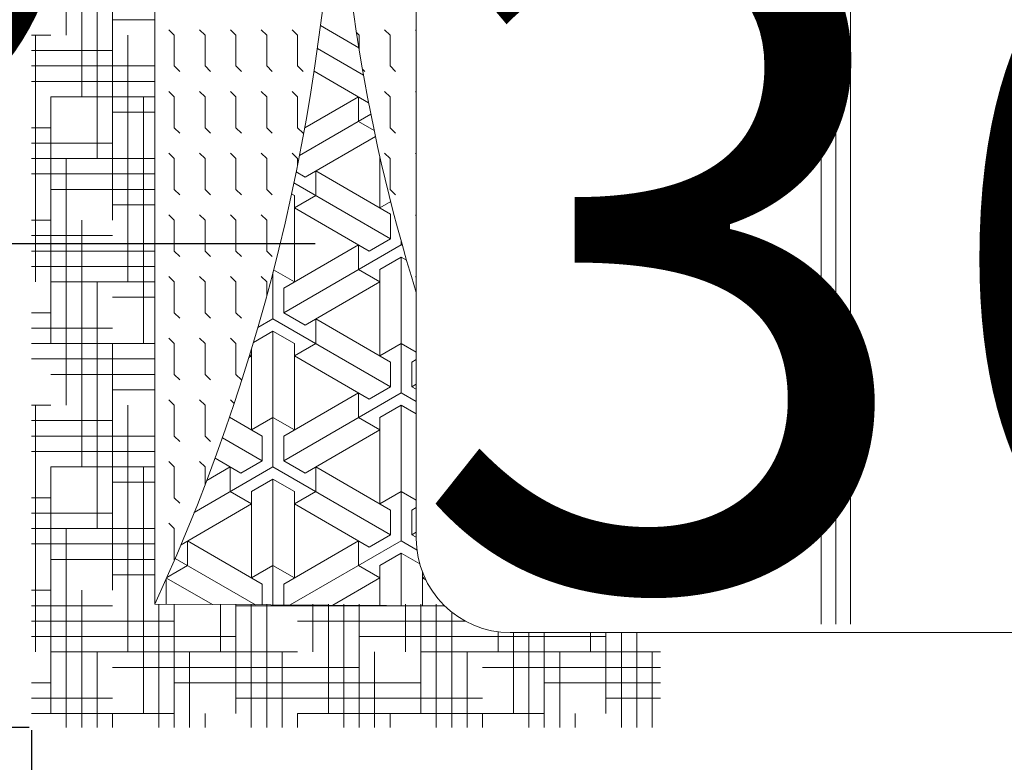
# Model space of a CAD drawing. Units: inches. Extents: x -90 to 536, y -553 to 299.
# Tile 5 of 27: x 96 to 122, y -394 to -375. Entities that reach past the tile are written whole.
import ezdxf

# ---------------------------------------------------------------- set-up
doc = ezdxf.new("R2010")
doc.units = ezdxf.units.IN
doc.layers.add('A-ANNO-DIMS', color=2, linetype='Continuous', lineweight=18)
doc.layers.add('Furniture', color=2, linetype='Continuous', lineweight=18)
doc.styles.get("Standard").update_dxf_attribs({"font": 'arial.ttf'})
doc.dimstyles.get("Standard").update_dxf_attribs({"dimtxt": 18, "dimasz": 12, "dimexe": 0.18, "dimexo": 0.0625, "dimgap": 0.09, "dimtad": 0, "dimtih": 1, "dimtoh": 1, "dimdec": 0, "dimzin": 0, "dimdsep": 46, "dimlunit": 3, "dimtxsty": 'Standard', "dimcen": 0.09, "dimadec": 0, "dimazin": 0, "dimtfac": 1, "dimtdec": 0, "dimtofl": 0, "dimtmove": 0, "dimatfit": 3, "dimfxl": 1, "dimtolj": 1, "dimtzin": 0, "dimarcsym": 0})

# ---------------------------------------------------------------- blocks, each defined once
blk = doc.blocks.new('A$C62731D1C')
for p, q in [((1.46787, 2.14084, 0.68571), (1.46787, 0.38824, 0.68571)), ((0.10613, 0.66415, 0.68571), (1.46095, 0.66415, 0.68571)), ((0.10613, 0.65215, 0.68571), (1.46095, 0.65215, 0.68571)), ((0.10613, 0.64015, 0.68571), (1.46095, 0.64015, 0.68571)), ((1.4835, 0.31577, 0.68571), (1.4835, 0.50998, 0.68571)), ((1.4835, 0.50327, 0.68571), (1.54488, 0.50327, 0.68571)), ((1.496, 0.36577, 0.68571), (1.496, 0.50998, 0.68571)), ((1.5085, 0.41577, 0.68571), (1.5085, 0.50998, 0.68571)), ((1.521, 0.46577, 0.68571), (1.521, 0.50998, 0.68571)), ((1.46787, 0.49077, 0.68571), (1.54488, 0.49077, 0.68571)), ((1.46787, 0.47827, 0.68571), (1.54488, 0.47827, 0.68571)), ((1.46787, 0.46577, 0.68571), (1.5335, 0.46577, 0.68571)), ((1.471, 0.26577, 0.68571), (1.471, 0.46577, 0.68571)), ((1.46787, 0.45327, 0.68571), (1.4835, 0.45327, 0.68571)), ((1.5335, 0.44077, 0.68571), (1.54488, 0.44077, 0.68571)), ((1.4835, 0.42827, 0.68571), (1.54488, 0.42827, 0.68571)), ((1.46787, 0.41577, 0.68571), (1.54488, 0.41577, 0.68571)), ((1.5335, 0.21577, 0.68571), (1.5335, 0.41577, 0.68571)), ((1.46787, 0.40327, 0.68571), (1.54488, 0.40327, 0.68571)), ((1.46787, 0.39077, 0.68571), (1.5335, 0.39077, 0.68571)), ((1.46722, 0.37827, 0.68571), (1.4835, 0.37827, 0.68571)), ((1.521, 0.16577, 0.68571), (1.521, 0.36577, 0.68571)), ((1.5335, 0.36577, 0.68571), (1.54488, 0.36577, 0.68571)), ((1.4585, 0.21577, 0.68571), (1.4585, 0.35163, 0.68571)), ((1.4835, 0.35327, 0.68571), (1.54488, 0.35327, 0.68571)), ((1.45128, 0.34077, 0.68571), (1.54488, 0.34077, 0.68571)), ((1.446, 0.33481, 0.68571), (1.44488, 0.1, 0.68571)), ((1.44488, 0.32827, 0.68571), (1.54488, 0.32827, 0.68571)), ((1.446, 0.16577, 0.68571), (1.446, 0.33481, 0.68571)), ((1.42502, 0.31973, 0.68571), (1.4235, 0.31709, 0.68571)), ((1.39167, 0.31204, 0.68571), (0.17247, 0.31204, 0.68571)), ((0.97908, 0.31135, 0.68571), (0.97977, 0.31204, 0.68571)), ((1.02908, 0.31135, 0.68571), (1.02977, 0.31204, 0.68571)), ((1.07908, 0.31135, 0.68571), (1.07977, 0.31204, 0.68571)), ((1.12908, 0.31135, 0.68571), (1.12977, 0.31204, 0.68571)), ((1.17908, 0.31135, 0.68571), (1.17977, 0.31204, 0.68571)), ((1.2335, 0.29977, 0.68571), (1.24058, 0.31204, 0.68571)), ((1.2485, 0.30843, 0.68571), (1.24642, 0.31204, 0.68571)), ((1.26642, 0.31204, 0.68571), (1.2685, 0.30843, 0.68571)), ((1.2685, 0.30843, 0.68571), (1.27058, 0.31204, 0.68571)), ((1.2735, 0.29977, 0.68571), (1.28058, 0.31204, 0.68571)), ((1.2835, 0.29977, 0.68571), (1.29058, 0.31204, 0.68571)), ((1.3535, 0.29977, 0.68571), (1.36058, 0.31204, 0.68571)), ((1.3685, 0.30843, 0.68571), (1.36642, 0.31204, 0.68571)), ((1.38642, 0.31204, 0.68571), (1.3885, 0.30843, 0.68571)), ((1.3885, 0.30843, 0.68571), (1.39058, 0.31204, 0.68571)), ((1.3935, 0.29977, 0.68571), (1.40091, 0.3126, 0.68571)), ((1.4035, 0.29977, 0.68571), (1.41221, 0.31486, 0.68571)), ((1.41896, 0.31709, 0.68571), (1.44592, 0.31709, 0.68571)), ((1.42263, 0.31861, 0.68571), (1.4235, 0.31709, 0.68571)), ((1.44488, 0.31577, 0.68571), (1.5335, 0.31577, 0.68571)), ((1.5085, 0.11577, 0.68571), (1.5085, 0.31577, 0.68571)), ((1.1635, 0.29977, 0.68571), (1.16604, 0.30418, 0.68571)), ((1.2685, 0.30843, 0.68571), (1.2485, 0.30843, 0.68571)), ((1.3885, 0.30843, 0.68571), (1.3685, 0.30843, 0.68571)), ((1.1535, 0.29977, 0.68571), (1.15051, 0.29977, 0.68571)), ((1.1535, 0.29977, 0.68571), (1.15408, 0.30077, 0.68571)), ((1.1535, 0.29977, 0.68571), (1.2085, 0.20451, 0.68571)), ((1.2735, 0.29977, 0.68571), (1.1635, 0.29977, 0.68571)), ((1.1635, 0.29977, 0.68571), (1.1735, 0.28245, 0.68571)), ((1.2335, 0.29977, 0.68571), (1.2435, 0.28245, 0.68571)), ((1.2735, 0.29977, 0.68571), (1.3285, 0.20451, 0.68571)), ((1.3935, 0.29977, 0.68571), (1.2835, 0.29977, 0.68571)), ((1.2835, 0.29977, 0.68571), (1.2935, 0.28245, 0.68571)), ((1.3535, 0.29977, 0.68571), (1.3635, 0.28245, 0.68571)), ((1.3935, 0.29977, 0.68571), (1.44541, 0.20987, 0.68571)), ((1.44583, 0.29977, 0.68571), (1.4035, 0.29977, 0.68571)), ((1.4035, 0.29977, 0.68571), (1.4135, 0.28245, 0.68571)), ((1.44488, 0.30327, 0.68571), (1.4835, 0.30327, 0.68571)), ((0.97908, 0.28635, 0.68571), (0.9835, 0.29077, 0.68571)), ((0.9835, 0.29077, 0.68571), (1.0085, 0.29077, 0.68571)), ((1.0085, 0.29077, 0.68571), (1.01292, 0.29519, 0.68571)), ((1.02908, 0.28635, 0.68571), (1.0335, 0.29077, 0.68571)), ((1.0335, 0.29077, 0.68571), (1.0585, 0.29077, 0.68571)), ((1.0585, 0.29077, 0.68571), (1.06292, 0.29519, 0.68571)), ((1.07908, 0.28635, 0.68571), (1.0835, 0.29077, 0.68571)), ((1.0835, 0.29077, 0.68571), (1.1085, 0.29077, 0.68571)), ((1.1285, 0.29111, 0.68571), (1.0935, 0.23049, 0.68571)), ((1.10332, 0.21286, 0.68571), (1.1485, 0.29111, 0.68571)), ((1.1085, 0.29077, 0.68571), (1.11292, 0.29519, 0.68571)), ((1.11842, 0.29126, 0.68571), (1.1235, 0.28245, 0.68571)), ((1.1485, 0.29111, 0.68571), (1.1285, 0.29111, 0.68571)), ((1.1485, 0.29111, 0.68571), (1.1585, 0.27379, 0.68571)), ((1.2135, 0.19585, 0.68571), (1.2685, 0.29111, 0.68571)), ((1.2485, 0.29111, 0.68571), (1.2135, 0.23049, 0.68571)), ((1.2685, 0.29111, 0.68571), (1.2485, 0.29111, 0.68571)), ((1.2685, 0.29111, 0.68571), (1.2785, 0.27379, 0.68571)), ((1.3335, 0.19585, 0.68571), (1.3885, 0.29111, 0.68571)), ((1.3685, 0.29111, 0.68571), (1.3335, 0.23049, 0.68571)), ((1.3885, 0.29111, 0.68571), (1.3685, 0.29111, 0.68571)), ((1.3885, 0.29111, 0.68571), (1.3985, 0.27379, 0.68571)), ((1.5335, 0.29077, 0.68571), (1.54488, 0.29077, 0.68571)), ((1.08156, 0.28245, 0.68571), (1.1235, 0.28245, 0.68571)), ((1.1735, 0.26513, 0.68571), (1.1835, 0.28245, 0.68571)), ((1.1735, 0.28245, 0.68571), (1.2435, 0.28245, 0.68571)), ((1.2185, 0.22183, 0.68571), (1.1835, 0.28245, 0.68571)), ((1.2935, 0.26513, 0.68571), (1.3035, 0.28245, 0.68571)), ((1.2935, 0.28245, 0.68571), (1.3635, 0.28245, 0.68571)), ((1.3385, 0.22183, 0.68571), (1.3035, 0.28245, 0.68571)), ((1.4135, 0.26513, 0.68571), (1.4235, 0.28245, 0.68571)), ((1.4135, 0.28245, 0.68571), (1.44575, 0.28245, 0.68571)), ((1.44557, 0.24423, 0.68571), (1.4235, 0.28245, 0.68571)), ((1.03828, 0.2734, 0.68571), (1.01275, 0.2292, 0.68571)), ((1.04766, 0.27525, 0.68571), (1.08108, 0.21737, 0.68571)), ((1.0535, 0.26513, 0.68571), (1.06091, 0.27796, 0.68571)), ((1.0985, 0.22183, 0.68571), (1.06553, 0.27894, 0.68571)), ((1.1585, 0.27379, 0.68571), (1.1235, 0.21317, 0.68571)), ((1.2785, 0.27379, 0.68571), (1.2435, 0.21317, 0.68571)), ((1.3985, 0.27379, 0.68571), (1.3635, 0.21317, 0.68571)), ((1.4835, 0.27827, 0.68571), (1.54488, 0.27827, 0.68571)), ((0.99372, 0.26552, 0.68571), (0.97573, 0.23435, 0.68571)), ((0.98131, 0.26358, 0.68571), (0.9835, 0.26577, 0.68571)), ((0.9835, 0.26577, 0.68571), (0.99527, 0.26577, 0.68571)), ((0.9943, 0.23188, 0.68571), (1.01588, 0.26926, 0.68571)), ((1.01117, 0.26843, 0.68571), (1.01292, 0.27019, 0.68571)), ((1.0535, 0.26513, 0.68571), (1.0335, 0.26513, 0.68571)), ((1.05864, 0.22159, 0.68571), (1.0335, 0.26513, 0.68571)), ((1.1735, 0.26513, 0.68571), (1.1535, 0.26513, 0.68571)), ((1.1885, 0.20451, 0.68571), (1.1535, 0.26513, 0.68571)), ((1.2935, 0.26513, 0.68571), (1.2735, 0.26513, 0.68571)), ((1.3085, 0.20451, 0.68571), (1.2735, 0.26513, 0.68571)), ((1.4135, 0.26513, 0.68571), (1.3935, 0.26513, 0.68571)), ((1.4285, 0.20451, 0.68571), (1.3935, 0.26513, 0.68571)), ((1.44488, 0.26577, 0.68571), (1.54488, 0.26577, 0.68571)), ((1.496, 0.06577, 0.68571), (1.496, 0.26577, 0.68571)), ((1.44488, 0.25327, 0.68571), (1.54488, 0.25327, 0.68571)), ((1.44488, 0.24077, 0.68571), (1.5335, 0.24077, 0.68571)), ((1.1135, 0.23049, 0.68571), (1.0935, 0.23049, 0.68571)), ((1.1135, 0.23049, 0.68571), (1.1235, 0.21317, 0.68571)), ((1.2335, 0.23049, 0.68571), (1.2135, 0.23049, 0.68571)), ((1.2335, 0.23049, 0.68571), (1.2435, 0.21317, 0.68571)), ((1.3535, 0.23049, 0.68571), (1.3335, 0.23049, 0.68571)), ((1.3535, 0.23049, 0.68571), (1.3635, 0.21317, 0.68571)), ((1.44488, 0.22827, 0.68571), (1.4835, 0.22827, 0.68571)), ((0.97908, 0.21135, 0.68571), (0.9835, 0.21577, 0.68571)), ((0.9835, 0.21577, 0.68571), (1.0085, 0.21577, 0.68571)), ((1.0085, 0.21577, 0.68571), (1.01292, 0.22019, 0.68571)), ((1.02908, 0.21135, 0.68571), (1.0335, 0.21577, 0.68571)), ((1.0335, 0.21577, 0.68571), (1.0585, 0.21577, 0.68571)), ((1.0585, 0.21577, 0.68571), (1.06292, 0.22019, 0.68571)), ((1.07908, 0.21135, 0.68571), (1.0835, 0.21577, 0.68571)), ((1.0835, 0.21577, 0.68571), (1.08915, 0.21577, 0.68571)), ((1.09439, 0.21471, 0.68571), (1.0985, 0.22183, 0.68571)), ((1.2085, 0.20451, 0.68571), (1.2185, 0.22183, 0.68571)), ((1.3285, 0.20451, 0.68571), (1.3385, 0.22183, 0.68571)), ((1.4835, 0.01577, 0.68571), (1.4835, 0.21577, 0.68571)), ((1.5335, 0.21577, 0.68571), (1.54488, 0.21577, 0.68571)), ((1.11222, 0.21096, 0.68571), (1.1135, 0.21317, 0.68571)), ((1.1135, 0.21317, 0.68571), (1.1835, 0.21317, 0.68571)), ((1.17381, 0.19638, 0.68571), (1.1835, 0.21317, 0.68571)), ((1.2235, 0.19585, 0.68571), (1.2335, 0.21317, 0.68571)), ((1.2335, 0.21317, 0.68571), (1.3035, 0.21317, 0.68571)), ((1.2935, 0.19585, 0.68571), (1.3035, 0.21317, 0.68571)), ((1.3435, 0.19585, 0.68571), (1.3535, 0.21317, 0.68571)), ((1.3535, 0.21317, 0.68571), (1.4235, 0.21317, 0.68571)), ((1.4135, 0.19585, 0.68571), (1.4235, 0.21317, 0.68571)), ((1.2085, 0.20451, 0.68571), (1.1885, 0.20451, 0.68571)), ((1.3285, 0.20451, 0.68571), (1.3085, 0.20451, 0.68571)), ((1.44538, 0.20451, 0.68571), (1.4285, 0.20451, 0.68571)), ((1.4835, 0.20327, 0.68571), (1.54488, 0.20327, 0.68571)), ((1.0085, 0.19077, 0.68571), (1.01292, 0.19519, 0.68571)), ((1.0585, 0.19077, 0.68571), (1.06292, 0.19519, 0.68571)), ((1.1085, 0.19077, 0.68571), (1.11292, 0.19519, 0.68571)), ((1.1585, 0.19077, 0.68571), (1.16292, 0.19519, 0.68571)), ((1.2135, 0.19585, 0.68571), (1.17586, 0.19585, 0.68571)), ((1.2135, 0.19585, 0.68571), (1.22059, 0.18358, 0.68571)), ((1.3335, 0.19585, 0.68571), (1.2235, 0.19585, 0.68571)), ((1.2235, 0.19585, 0.68571), (1.23263, 0.18003, 0.68571)), ((1.2935, 0.19585, 0.68571), (1.3035, 0.17853, 0.68571)), ((1.3335, 0.19585, 0.68571), (1.37035, 0.13204, 0.68571)), ((1.44534, 0.19585, 0.68571), (1.3435, 0.19585, 0.68571)), ((1.3435, 0.19585, 0.68571), (1.3535, 0.17853, 0.68571)), ((1.4135, 0.19585, 0.68571), (1.4235, 0.17853, 0.68571)), ((0.97908, 0.18635, 0.68571), (0.9835, 0.19077, 0.68571)), ((0.9835, 0.19077, 0.68571), (1.0085, 0.19077, 0.68571)), ((1.02908, 0.18635, 0.68571), (1.0335, 0.19077, 0.68571)), ((1.0335, 0.19077, 0.68571), (1.0585, 0.19077, 0.68571)), ((1.07908, 0.18635, 0.68571), (1.0835, 0.19077, 0.68571)), ((1.0835, 0.19077, 0.68571), (1.1085, 0.19077, 0.68571)), ((1.12908, 0.18635, 0.68571), (1.1335, 0.19077, 0.68571)), ((1.1335, 0.19077, 0.68571), (1.1585, 0.19077, 0.68571)), ((1.17908, 0.18635, 0.68571), (1.1835, 0.19077, 0.68571)), ((1.1835, 0.19077, 0.68571), (1.195, 0.19077, 0.68571)), ((1.2085, 0.18719, 0.68571), (1.20794, 0.18719, 0.68571)), ((1.20842, 0.18705, 0.68571), (1.2085, 0.18719, 0.68571)), ((1.2085, 0.18719, 0.68571), (1.20861, 0.187, 0.68571)), ((1.3085, 0.18719, 0.68571), (1.29318, 0.16065, 0.68571)), ((1.3285, 0.18719, 0.68571), (1.3085, 0.18719, 0.68571)), ((1.30983, 0.15486, 0.68571), (1.3285, 0.18719, 0.68571)), ((1.3285, 0.18719, 0.68571), (1.3385, 0.16987, 0.68571)), ((1.4285, 0.18719, 0.68571), (1.3935, 0.12657, 0.68571)), ((1.4453, 0.18719, 0.68571), (1.4285, 0.18719, 0.68571)), ((1.44488, 0.19077, 0.68571), (1.54488, 0.19077, 0.68571)), ((1.23764, 0.17853, 0.68571), (1.3035, 0.17853, 0.68571)), ((1.24263, 0.17702, 0.68571), (1.2435, 0.17853, 0.68571)), ((1.24475, 0.17637, 0.68571), (1.2435, 0.17853, 0.68571)), ((1.3535, 0.16121, 0.68571), (1.3635, 0.17853, 0.68571)), ((1.3535, 0.17853, 0.68571), (1.4235, 0.17853, 0.68571)), ((1.39656, 0.12128, 0.68571), (1.3635, 0.17853, 0.68571)), ((1.40771, 0.11653, 0.68571), (1.44527, 0.1816, 0.68571)), ((1.44488, 0.17827, 0.68571), (1.54488, 0.17827, 0.68571)), ((1.0085, 0.16577, 0.68571), (1.01292, 0.17019, 0.68571)), ((1.0585, 0.16577, 0.68571), (1.06292, 0.17019, 0.68571)), ((1.1085, 0.16577, 0.68571), (1.11292, 0.17019, 0.68571)), ((1.1585, 0.16577, 0.68571), (1.16292, 0.17019, 0.68571)), ((1.2085, 0.16577, 0.68571), (1.21292, 0.17019, 0.68571)), ((1.2585, 0.16577, 0.68571), (1.26292, 0.17019, 0.68571)), ((1.3385, 0.16987, 0.68571), (1.32639, 0.14889, 0.68571)), ((0.97908, 0.16135, 0.68571), (0.9835, 0.16577, 0.68571)), ((0.9835, 0.16577, 0.68571), (1.0085, 0.16577, 0.68571)), ((1.02908, 0.16135, 0.68571), (1.0335, 0.16577, 0.68571)), ((1.0335, 0.16577, 0.68571), (1.0585, 0.16577, 0.68571)), ((1.07908, 0.16135, 0.68571), (1.0835, 0.16577, 0.68571)), ((1.0835, 0.16577, 0.68571), (1.1085, 0.16577, 0.68571)), ((1.12908, 0.16135, 0.68571), (1.1335, 0.16577, 0.68571)), ((1.1335, 0.16577, 0.68571), (1.1585, 0.16577, 0.68571)), ((1.17908, 0.16135, 0.68571), (1.1835, 0.16577, 0.68571)), ((1.1835, 0.16577, 0.68571), (1.2085, 0.16577, 0.68571)), ((1.22908, 0.16135, 0.68571), (1.2335, 0.16577, 0.68571)), ((1.2335, 0.16577, 0.68571), (1.2585, 0.16577, 0.68571)), ((1.27908, 0.16135, 0.68571), (1.28212, 0.16439, 0.68571)), ((1.3535, 0.16121, 0.68571), (1.3335, 0.16121, 0.68571)), ((1.34453, 0.14211, 0.68571), (1.3335, 0.16121, 0.68571)), ((1.44488, 0.16577, 0.68571), (1.5335, 0.16577, 0.68571)), ((1.471, 0, 0.68571), (1.471, 0.16577, 0.68571)), ((1.44488, 0.15327, 0.68571), (1.4835, 0.15327, 0.68571)), ((1.0085, 0.14077, 0.68571), (1.01292, 0.14519, 0.68571)), ((1.0585, 0.14077, 0.68571), (1.06292, 0.14519, 0.68571)), ((1.1085, 0.14077, 0.68571), (1.11292, 0.14519, 0.68571)), ((1.1585, 0.14077, 0.68571), (1.16292, 0.14519, 0.68571)), ((1.2085, 0.14077, 0.68571), (1.21292, 0.14519, 0.68571)), ((1.2585, 0.14077, 0.68571), (1.26292, 0.14519, 0.68571)), ((1.3085, 0.14077, 0.68571), (1.31292, 0.14519, 0.68571)), ((1.44511, 0.14667, 0.68571), (1.42369, 0.10957, 0.68571)), ((0.97908, 0.13635, 0.68571), (0.9835, 0.14077, 0.68571)), ((0.9835, 0.14077, 0.68571), (1.0085, 0.14077, 0.68571)), ((1.02908, 0.13635, 0.68571), (1.0335, 0.14077, 0.68571)), ((1.0335, 0.14077, 0.68571), (1.0585, 0.14077, 0.68571)), ((1.07908, 0.13635, 0.68571), (1.0835, 0.14077, 0.68571)), ((1.0835, 0.14077, 0.68571), (1.1085, 0.14077, 0.68571)), ((1.12908, 0.13635, 0.68571), (1.1335, 0.14077, 0.68571)), ((1.1335, 0.14077, 0.68571), (1.1585, 0.14077, 0.68571)), ((1.17908, 0.13635, 0.68571), (1.1835, 0.14077, 0.68571)), ((1.1835, 0.14077, 0.68571), (1.2085, 0.14077, 0.68571)), ((1.22908, 0.13635, 0.68571), (1.2335, 0.14077, 0.68571)), ((1.2335, 0.14077, 0.68571), (1.2585, 0.14077, 0.68571)), ((1.27908, 0.13635, 0.68571), (1.2835, 0.14077, 0.68571)), ((1.2835, 0.14077, 0.68571), (1.3085, 0.14077, 0.68571)), ((1.32908, 0.13635, 0.68571), (1.3335, 0.14077, 0.68571)), ((1.3335, 0.14077, 0.68571), (1.34805, 0.14077, 0.68571)), ((1.5335, 0.14077, 0.68571), (1.54488, 0.14077, 0.68571)), ((1.4835, 0.12827, 0.68571), (1.54488, 0.12827, 0.68571)), ((1.0085, 0.11577, 0.68571), (1.01292, 0.12019, 0.68571)), ((1.0585, 0.11577, 0.68571), (1.06292, 0.12019, 0.68571)), ((1.1085, 0.11577, 0.68571), (1.11292, 0.12019, 0.68571)), ((1.1585, 0.11577, 0.68571), (1.16292, 0.12019, 0.68571)), ((1.2085, 0.11577, 0.68571), (1.21292, 0.12019, 0.68571)), ((1.2585, 0.11577, 0.68571), (1.26292, 0.12019, 0.68571)), ((1.3085, 0.11577, 0.68571), (1.31292, 0.12019, 0.68571)), ((1.3585, 0.11577, 0.68571), (1.36292, 0.12019, 0.68571)), ((1.4135, 0.12657, 0.68571), (1.3935, 0.12657, 0.68571)), ((1.4135, 0.12657, 0.68571), (1.42319, 0.10978, 0.68571)), ((0.97908, 0.11135, 0.68571), (0.9835, 0.11577, 0.68571)), ((0.9835, 0.11577, 0.68571), (1.0085, 0.11577, 0.68571)), ((1.02908, 0.11135, 0.68571), (1.0335, 0.11577, 0.68571)), ((1.0335, 0.11577, 0.68571), (1.0585, 0.11577, 0.68571)), ((1.07908, 0.11135, 0.68571), (1.0835, 0.11577, 0.68571)), ((1.0835, 0.11577, 0.68571), (1.1085, 0.11577, 0.68571)), ((1.12908, 0.11135, 0.68571), (1.1335, 0.11577, 0.68571)), ((1.1335, 0.11577, 0.68571), (1.1585, 0.11577, 0.68571)), ((1.17908, 0.11135, 0.68571), (1.1835, 0.11577, 0.68571)), ((1.1835, 0.11577, 0.68571), (1.2085, 0.11577, 0.68571)), ((1.22908, 0.11135, 0.68571), (1.2335, 0.11577, 0.68571)), ((1.2335, 0.11577, 0.68571), (1.2585, 0.11577, 0.68571)), ((1.27908, 0.11135, 0.68571), (1.2835, 0.11577, 0.68571)), ((1.2835, 0.11577, 0.68571), (1.3085, 0.11577, 0.68571)), ((1.32908, 0.11135, 0.68571), (1.3335, 0.11577, 0.68571)), ((1.3335, 0.11577, 0.68571), (1.3585, 0.11577, 0.68571)), ((1.37908, 0.11135, 0.68571), (1.3835, 0.11577, 0.68571)), ((1.3835, 0.11577, 0.68571), (1.4085, 0.11577, 0.68571)), ((1.4085, 0.11577, 0.68571), (1.4088, 0.11607, 0.68571)), ((1.44488, 0.11577, 0.68571), (1.54488, 0.11577, 0.68571)), ((1.4585, 0, 0.68571), (1.4585, 0.11577, 0.68571)), ((1.5335, 0, 0.68571), (1.5335, 0.11577, 0.68571)), ((1.4244, 0.10925, 0.68571), (1.44493, 0.10925, 0.68571)), ((1.44488, 0.1, 0.68571), (0.1, 0.1, 0.68571)), ((0.971, 0.06577, 0.68571), (0.971, 0.1, 0.68571)), ((1.0085, 0, 0.68571), (1.0085, 0.1, 0.68571)), ((1.021, 0, 0.68571), (1.021, 0.1, 0.68571)), ((1.0335, 0.01577, 0.68571), (1.0335, 0.1, 0.68571)), ((1.046, 0.06577, 0.68571), (1.046, 0.1, 0.68571)), ((1.0835, 0, 0.68571), (1.0835, 0.1, 0.68571)), ((1.096, 0, 0.68571), (1.096, 0.1, 0.68571)), ((1.1085, 0.01577, 0.68571), (1.1085, 0.1, 0.68571)), ((1.121, 0.06577, 0.68571), (1.121, 0.1, 0.68571)), ((1.1585, 0, 0.68571), (1.1585, 0.1, 0.68571)), ((1.171, 0, 0.68571), (1.171, 0.1, 0.68571)), ((1.1835, 0.01577, 0.68571), (1.1835, 0.1, 0.68571)), ((1.196, 0.06577, 0.68571), (1.196, 0.1, 0.68571)), ((1.2335, 0, 0.68571), (1.2335, 0.1, 0.68571)), ((1.246, 0, 0.68571), (1.246, 0.1, 0.68571)), ((1.2585, 0.01577, 0.68571), (1.2585, 0.1, 0.68571)), ((1.271, 0.06577, 0.68571), (1.271, 0.1, 0.68571)), ((1.3085, 0, 0.68571), (1.3085, 0.1, 0.68571)), ((1.321, 0, 0.68571), (1.321, 0.1, 0.68571)), ((1.3335, 0.01577, 0.68571), (1.3335, 0.1, 0.68571)), ((1.346, 0.06577, 0.68571), (1.346, 0.1, 0.68571)), ((1.3835, 0, 0.68571), (1.3835, 0.1, 0.68571)), ((1.396, 0, 0.68571), (1.396, 0.1, 0.68571)), ((1.4085, 0.01577, 0.68571), (1.4085, 0.1, 0.68571)), ((1.421, 0.06577, 0.68571), (1.421, 0.1, 0.68571)), ((1.44488, 0.10327, 0.68571), (1.54488, 0.10327, 0.68571)), ((1.0335, 0.09077, 0.68571), (1.2335, 0.09077, 0.68571)), ((1.3335, 0.09077, 0.68571), (1.5335, 0.09077, 0.68571)), ((0.9835, 0.07827, 0.68571), (1.1835, 0.07827, 0.68571)), ((1.2835, 0.07827, 0.68571), (1.4835, 0.07827, 0.68571)), ((0.9335, 0.06577, 0.68571), (1.1335, 0.06577, 0.68571)), ((0.996, 0, 0.68571), (0.996, 0.06577, 0.68571)), ((1.071, 0, 0.68571), (1.071, 0.06577, 0.68571)), ((1.146, 0, 0.68571), (1.146, 0.06577, 0.68571)), ((1.221, 0, 0.68571), (1.221, 0.06577, 0.68571)), ((1.2335, 0.06577, 0.68571), (1.4335, 0.06577, 0.68571)), ((1.296, 0, 0.68571), (1.296, 0.06577, 0.68571)), ((1.371, 0, 0.68571), (1.371, 0.06577, 0.68571)), ((1.446, 0, 0.68571), (1.446, 0.06577, 0.68571)), ((1.521, 0, 0.68571), (1.521, 0.06577, 0.68571)), ((1.5335, 0.06577, 0.68571), (1.54488, 0.06577, 0.68571)), ((0.8835, 0.05327, 0.68571), (1.0835, 0.05327, 0.68571)), ((1.1835, 0.05327, 0.68571), (1.3835, 0.05327, 0.68571)), ((1.4835, 0.05327, 0.68571), (1.54488, 0.05327, 0.68571)), ((0.8335, 0.04077, 0.68571), (1.0335, 0.04077, 0.68571)), ((1.1335, 0.04077, 0.68571), (1.3335, 0.04077, 0.68571)), ((1.4335, 0.04077, 0.68571), (1.54488, 0.04077, 0.68571)), ((0.7835, 0.02827, 0.68571), (0.9835, 0.02827, 0.68571)), ((1.0835, 0.02827, 0.68571), (1.2835, 0.02827, 0.68571)), ((1.3835, 0.02827, 0.68571), (1.54488, 0.02827, 0.68571)), ((0.9835, 0, 0.68571), (0.9835, 0.01577, 0.68571)), ((1.0335, 0.01577, 0.68571), (1.2335, 0.01577, 0.68571)), ((1.0585, 0, 0.68571), (1.0585, 0.01577, 0.68571)), ((1.1335, 0, 0.68571), (1.1335, 0.01577, 0.68571)), ((1.2085, 0, 0.68571), (1.2085, 0.01577, 0.68571)), ((1.2835, 0, 0.68571), (1.2835, 0.01577, 0.68571)), ((1.3335, 0.01577, 0.68571), (1.5335, 0.01577, 0.68571)), ((1.3585, 0, 0.68571), (1.3585, 0.01577, 0.68571)), ((1.4335, 0, 0.68571), (1.4335, 0.01577, 0.68571)), ((1.5085, 0, 0.68571), (1.5085, 0.01577, 0.68571)), ((0.9835, 0.00327, 0.68571), (1.1835, 0.00327, 0.68571)), ((1.2835, 0.00327, 0.68571), (1.4835, 0.00327, 0.68571))]:
    blk.add_line(p, q)
for centre, radius, start, end in [((1.39167, 0.38824, 0.68571), 0.0762, 270, 0), ((0.76456, 1.69033, 0.68571), 1.44313, 252.76056, 287.23944), ((0.77244, -1.36185, 0.68571), 1.6091, 65.29791, 114.70209)]:
    blk.add_arc(centre, radius, start, end)
blk = doc.blocks.new('A$C0E6D7E3D')
blk.add_blockref('A$C62731D1C', (0, 0))
blk = doc.blocks.new('*D27')
at = {"layer": 'A-ANNO-DIMS', "color": 0, "lineweight": -2, "transparency": 16777216}
for p, q in [((49.132, -428.616), (49.132, -434.359)), ((86.632, -428.616), (86.632, -434.359)), ((61.132, -434.179), (74.632, -434.179)), ((86.632, -434.179), (98.632, -434.179))]:
    blk.add_line(p, q, dxfattribs=at)
at = {"layer": 'A-ANNO-DIMS', "color": 0, "transparency": 16777216}
for points in [[(61.132, -432.179), (61.132, -436.179), (49.132, -434.179)], [(74.632, -432.179), (74.632, -436.179), (86.632, -434.179)]]:
    blk.add_solid(points, dxfattribs=at)
at = {"layer": 'Defpoints', "color": 0, "transparency": 16777216}
for p in [(49.132, -428.554), (86.632, -428.554), (86.632, -434.179)]:
    blk.add_point(p, dxfattribs=at)
at = {"layer": 'A-ANNO-DIMS', "color": 0, "transparency": 16777216, "insert": (195.174, -434.179), "char_height": 18, "attachment_point": 5}
blk.add_mtext('\\A1;DOOR B 38 TYP.', dxfattribs=at)
blk = doc.blocks.new('*D28')
at = {"layer": 'A-ANNO-DIMS', "color": 0, "lineweight": -2, "transparency": 16777216}
for p, q in [((92.257, -392.554), (92.257, -380.554)), ((92.257, -380.554), (104.257, -380.554)), ((86.694, -392.554), (92.437, -392.554)), ((92.257, -416.554), (92.257, -404.554)), ((86.694, -428.554), (92.437, -428.554))]:
    blk.add_line(p, q, dxfattribs=at)
at = {"layer": 'A-ANNO-DIMS', "color": 0, "transparency": 16777216}
for points in [[(90.257, -404.554), (94.257, -404.554), (92.257, -392.554)], [(90.257, -416.554), (94.257, -416.554), (92.257, -428.554)]]:
    blk.add_solid(points, dxfattribs=at)
at = {"layer": 'Defpoints', "color": 0, "transparency": 16777216}
for p in [(86.632, -392.554), (92.257, -392.554), (86.632, -428.554)]:
    blk.add_point(p, dxfattribs=at)
at = {"layer": 'A-ANNO-DIMS', "color": 0, "transparency": 16777216, "insert": (148.15, -380.554), "char_height": 18, "attachment_point": 5}
blk.add_mtext('\\A1;36 TYP.', dxfattribs=at)
blk = doc.blocks.new('*D51')
at = {"layer": 'A-ANNO-DIMS', "color": 0, "lineweight": -2, "transparency": 16777216}
for p, q in [((96.806, -393.34), (96.806, -404.606)), ((171.132, -393.34), (171.132, -404.606)), ((108.806, -404.426), (159.132, -404.426)), ((171.132, -404.426), (183.132, -404.426))]:
    blk.add_line(p, q, dxfattribs=at)
at = {"layer": 'A-ANNO-DIMS', "color": 0, "transparency": 16777216}
for points in [[(108.806, -402.426), (108.806, -406.426), (96.806, -404.426)], [(159.132, -402.426), (159.132, -406.426), (171.132, -404.426)]]:
    blk.add_solid(points, dxfattribs=at)
at = {"layer": 'Defpoints', "color": 0, "transparency": 16777216}
for p in [(96.806, -393.277), (171.132, -393.277), (171.132, -404.426)]:
    blk.add_point(p, dxfattribs=at)
at = {"layer": 'A-ANNO-DIMS', "color": 0, "transparency": 16777216, "insert": (274.99, -404.426), "char_height": 18, "attachment_point": 5}
blk.add_mtext('\\A1;SINGLE BED 74', dxfattribs=at)
blk = doc.blocks.new('*D52')
at = {"layer": 'A-ANNO-DIMS', "color": 0, "lineweight": -2, "transparency": 16777216}
for p, q in [((96.743, -343.206), (85.477, -343.206)), ((85.657, -355.206), (85.657, -358.961)), ((85.657, -381.277), (85.657, -377.522)), ((96.743, -393.277), (85.477, -393.277))]:
    blk.add_line(p, q, dxfattribs=at)
at = {"layer": 'A-ANNO-DIMS', "color": 0, "transparency": 16777216}
for points in [[(83.657, -355.206), (87.657, -355.206), (85.657, -343.206)], [(83.657, -381.277), (87.657, -381.277), (85.657, -393.277)]]:
    blk.add_solid(points, dxfattribs=at)
at = {"layer": 'Defpoints', "color": 0, "transparency": 16777216}
for p in [(96.806, -343.206), (85.657, -393.277), (96.806, -393.277)]:
    blk.add_point(p, dxfattribs=at)
at = {"layer": 'A-ANNO-DIMS', "color": 0, "transparency": 16777216, "insert": (85.657, -368.242), "char_height": 18, "attachment_point": 5}
blk.add_mtext('\\A1;50', dxfattribs=at)
blk = doc.blocks.new('*D54')
at = {"layer": 'A-ANNO-DIMS', "color": 0, "lineweight": -2, "transparency": 16777216}
for p, q in [((113.069, 249.446), (-2.848, 249.446)), ((-2.668, 237.446), (-2.668, -117.767)), ((-2.668, -491.554), (-2.668, -136.34)), ((38.069, -503.554), (-2.848, -503.554))]:
    blk.add_line(p, q, dxfattribs=at)
at = {"layer": 'A-ANNO-DIMS', "color": 0, "transparency": 16777216}
for points in [[(-4.668, 237.446), (-0.668, 237.446), (-2.668, 249.446)], [(-4.668, -491.554), (-0.668, -491.554), (-2.668, -503.554)]]:
    blk.add_solid(points, dxfattribs=at)
at = {"layer": 'Defpoints', "color": 0, "transparency": 16777216}
for p in [(-2.668, 249.446), (113.132, 249.446), (38.132, -503.554)]:
    blk.add_point(p, dxfattribs=at)
at = {"layer": 'A-ANNO-DIMS', "color": 0, "transparency": 16777216, "insert": (-2.668, -127.054), "char_height": 18, "attachment_point": 5}
blk.add_mtext('\\A1;753', dxfattribs=at)

msp = doc.modelspace()

# ---------------------------------------------------------------- block references
at = {"layer": 'Furniture', "xscale": 32.41097235378273, "yscale": 32.41097235378273, "zscale": 32.41097235378273, "rotation": 270}
msp.add_blockref('A$C0E6D7E3D', (96.8056, -343.2061, -22.2246), dxfattribs=at)

# ---------------------------------------------------------------- dimensions: what is measured, and where the dimension line sits
at = {"layer": 'A-ANNO-DIMS'}
for base, p1, p2, angle, picture, middle in [((-2.6677, 249.4462), (38.1317, -503.5538), (113.1317, 249.4462), 90, '*D54', (-2.6677, -127.0538)), ((85.6567, -393.2773), (96.8056, -343.2061), (96.8056, -393.2773), 270, '*D52', (85.6567, -368.2417))]:
    dim = msp.add_linear_dim(base=base, p1=p1, p2=p2, angle=angle, dimstyle='Standard', override={"dimdec": 0, "dimlfac": 1, "dimrnd": 0, "dimzin": 0, "dimdsep": 46, "dimlunit": 2}, dxfattribs=at)
    dim.commit()
    dim.dimension.update_dxf_attribs({"geometry": picture, "text_midpoint": middle})
dim = msp.add_linear_dim(base=(92.2567, -392.5538), p1=(86.6317, -428.5538), p2=(86.6317, -392.5538), angle=90, text='<> TYP.', dimstyle='Standard', override={"dimdec": 0, "dimlfac": 1, "dimrnd": 0, "dimzin": 0, "dimdsep": 46, "dimlunit": 2}, dxfattribs=at)
dim.commit()
dim.dimension.update_dxf_attribs({"geometry": '*D28', "text_midpoint": (148.1496, -380.5538)})
for base, p1, p2, text, picture, middle in [((171.1317, -404.4263), (96.8056, -393.2773), (171.1317, -393.2773), 'SINGLE BED <>', '*D51', (274.9898, -404.4263)), ((86.6317404714, -434.1787825705), (49.1317404714, -428.5537825705), (86.6317404714, -428.5537825705), 'DOOR B <> TYP.', '*D27', (195.1739914946, -434.1787825705))]:
    dim = msp.add_linear_dim(base=base, p1=p1, p2=p2, text=text, dimstyle='Standard', override={"dimdec": 0, "dimlfac": 1, "dimrnd": 0, "dimzin": 0, "dimdsep": 46, "dimlunit": 2}, dxfattribs=at)
    dim.commit()
    dim.dimension.update_dxf_attribs({"geometry": picture, "text_midpoint": middle})

doc.saveas('drawing.dxf')
